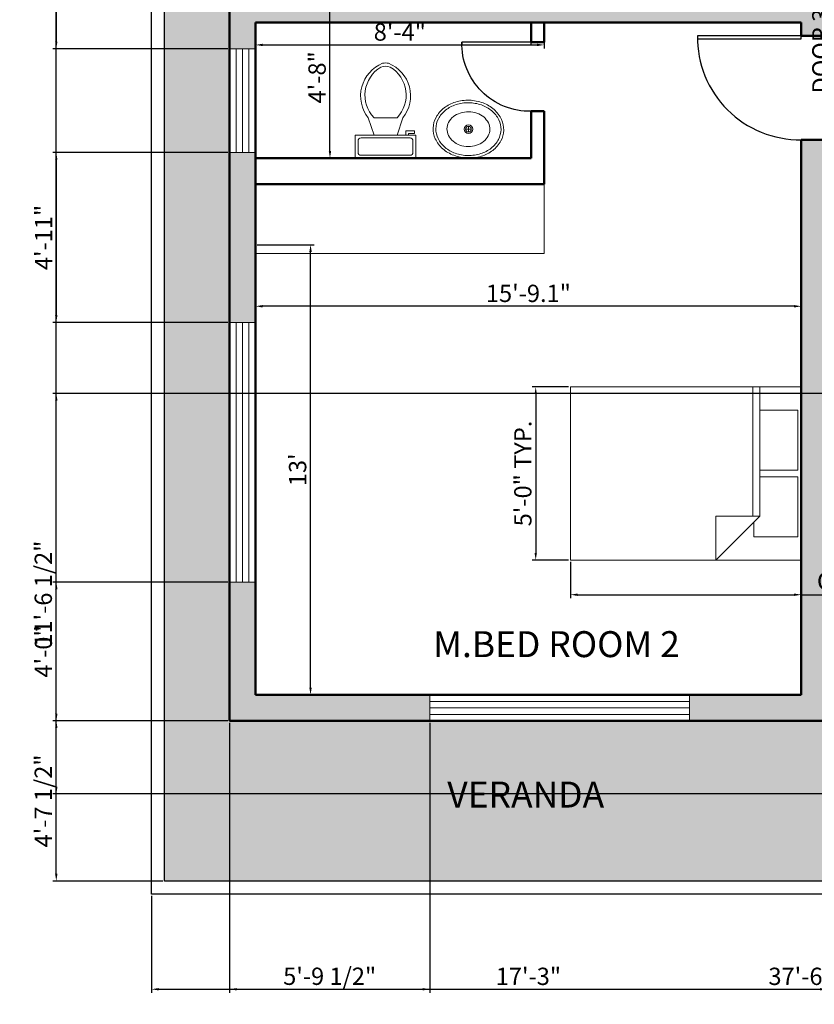
# Model space of a CAD drawing. Units: inches. Extents: x 2623 to 3157, y 1514 to 2273.
# Tile 1 of 6: x 2623 to 2898, y 1514 to 1856. Entities that reach past the tile are written whole.
import ezdxf

# ---------------------------------------------------------------- set-up
doc = ezdxf.new("R2010")
doc.units = ezdxf.units.IN
for name, color, linetype, lineweight in [('A-ANNO-DIMS', 2, 'Continuous', 18), ('A-AREA-IDEN', 7, 'Continuous', 25), ('A-DOOR', 4, 'Continuous', 25), ('A-FLOR-CASE', 8, 'Continuous', 20), ('A-FLOR-FIXT', 9, 'Continuous', 18), ('A-FURN', 8, 'Continuous', 18), ('A-GLAZ', 4, 'Continuous', 20), ('A-WALL', 7, 'Continuous', 50), ('A-WALL-PATT', 252, 'Continuous', 13), ('C-PROP', 7, 'Continuous', 25), ('L-PLNT-PATT', 9, 'Continuous', 13)]:
    doc.layers.add(name, color=color, linetype=linetype, lineweight=lineweight)
doc.styles.get("Standard").update_dxf_attribs({"font": 'arial.ttf'})
doc.dimstyles.new('ISO-25', dxfattribs={"dimtxt": 6, "dimasz": 2.5, "dimexe": 1.25, "dimexo": 0.625, "dimtad": 1, "dimdec": 1, "dimlunit": 3, "dimtxsty": 'Standard', "dimcen": 2.5, "dimadec": 0, "dimazin": 0, "dimtfac": 1, "dimtdec": 1, "dimtmove": 0, "dimatfit": 3, "dimfxl": 1, "dimarcsym": 0})

# ---------------------------------------------------------------- blocks, each defined once
blk = doc.blocks.new('Bed - Queen')
for p, q in [((0, -80.00003), (0, 0)), ((0, 0), (59.99999, 0)), ((59.99999, 0), (59.99999, -80.00003)), ((7.99999, -1.2), (28.79998, -1.2)), ((7.99999, -14.4), (7.99999, -1.2)), ((28.79998, -1.2), (28.79998, -14.4)), ((31.19999, -1.2), (51.99999, -1.2)), ((31.19999, -14.4), (31.19999, -1.2)), ((51.99999, -1.2), (51.99999, -16.4)), ((0, -14.4), (44.8, -14.4)), ((44.8, -16.8), (0, -16.8)), ((59.99999, -29.6), (44.8, -14.4)), ((44.8, -14.4), (44.8, -29.6)), ((51.99999, -16.4), (46.79936, -16.4)), ((44.8, -29.6), (59.99999, -29.6)), ((59.99999, -80.00003), (0, -80.00003))]:
    blk.add_line(p, q)
blk = doc.blocks.new('Toilet - top')
for p, q in [((9.5, -6), (9.5, -2)), ((-10, -8.5), (-8, -8.5)), ((-10, -9.5), (-10, -8.5)), ((-7, -9.5), (-10, -9.5)), ((-8, -8.5), (-8, -8)), ((-7, -8), (-7, -9.5)), ((-4, -8), (-6, -14)), ((4, -8), (6, -14)), ((4, -14), (-4, -14))]:
    blk.add_line(p, q)
blk.add_lwpolyline([(10.5, -8), (10.5, 0), (-10.5, 0), (-10.5, -8)], close=True)
for points in [[(-9.5, -2), (-9.5, -6)], [(8.5, -1), (-8.5, -1)], [(-8.5, -7), (8.5, -7)]]:
    blk.add_lwpolyline(points)
for centre, radius, start, end in [((-8.62, -1.88), 0.884, 81.8699, 188.1301), ((8.62, -1.88), 0.884, 351.8699, 98.1301), ((-8.62, -6.12), 0.884, 171.8699, 278.1301), ((8.62, -6.12), 0.884, 261.8699, 8.1301), ((3.52, -21.58), 12.17, 141.4691, 247.9714), ((4.2, -21.82), 11.33, 136.3677, 238.9468), ((-3.52, -21.58), 12.17, 292.0284, 38.5307), ((-4.2, -21.82), 11.33, 301.053, 43.6321), ((0, -27.88), 4, 245.7318, 294.2682), ((0, -29), 4, 254.8605, 285.1395)]:
    blk.add_arc(centre, radius, start, end)
blk = doc.blocks.new('Sink - Oval top')
for p, q in [((-1, 0), (1, 0)), ((0, 1), (0, -1))]:
    blk.add_line(p, q)
for points in [[(-12.23, 0.39, 0.117634), (-11.46, -3.36, 0.104469), (-8.88, -6.8, 0.090016), (-5.08, -9.07, 0.08192), (-0.32, -10.02, 0.08192), (4.49, -9.38, 0.090016), (8.42, -7.36, 0.104469), (11.22, -4.09, 0.117634), (12.23, -0.39, 0.117634), (11.46, 3.36, 0.104469), (8.88, 6.8, 0.090016), (5.08, 9.07, 0.08192), (0.32, 10.02, 0.08192), (-4.49, 9.38, 0.090016), (-8.42, 7.36, 0.104469), (-11.22, 4.09, 0.117634)], [(-11.29, 0.16, 0.118622), (-10.52, -3.25, 0.104678), (-8.07, -6.36, 0.089562), (-4.54, -8.37, 0.081185), (-0.13, -9.15, 0.081185), (4.3, -8.49, 0.089562), (7.89, -6.58, 0.104678), (10.42, -3.55, 0.118622), (11.29, -0.16, 0.118622), (10.52, 3.25, 0.104678), (8.07, 6.36, 0.089562), (4.54, 8.37, 0.081185), (0.13, 9.15, 0.081185), (-4.3, 8.49, 0.089562), (-7.89, 6.58, 0.104678), (-10.42, 3.55, 0.118622)], [(-7.42, 0.08, 0.118283), (-6.91, -2.17, 0.104607), (-5.29, -4.21, 0.089718), (-2.97, -5.53, 0.081436), (-0.07, -6.04, 0.081436), (2.84, -5.59, 0.089718), (5.2, -4.33, 0.104607), (6.86, -2.32, 0.118283), (7.42, -0.08, 0.118283), (6.91, 2.17, 0.104607), (5.29, 4.21, 0.089718), (2.97, 5.53, 0.081436), (0.07, 6.04, 0.081436), (-2.84, 5.59, 0.089718), (-5.2, 4.33, 0.104607), (-6.86, 2.32, 0.118283)]]:
    blk.add_lwpolyline(points, format="xyb", close=True)
for radius in [1.5, 1]:
    blk.add_circle((0, 0), radius)
blk = doc.blocks.new('Window - Wood Frame 36 in. Wide plan')
for p, q in [((0, 6), (0, 0)), ((36, 6), (36, 0)), ((0, 4.5), (36, 4.5)), ((0, 3), (36, 3)), ((0, 1.5), (36, 1.5))]:
    blk.add_line(p, q)
blk = doc.blocks.new('*D24')
at = {"layer": 'A-ANNO-DIMS', "color": 0, "lineweight": -2, "transparency": 16777216}
for p, q in [((2704.92, 1777.65), (2724.62, 1777.65)), ((2723.37, 1624.15), (2723.37, 1775.15)), ((2704.92, 1621.65), (2724.62, 1621.65))]:
    blk.add_line(p, q, dxfattribs=at)
at = {"layer": 'A-ANNO-DIMS', "color": 0, "transparency": 16777216}
for points in [[(2722.95, 1775.15), (2723.79, 1775.15), (2723.37, 1777.65)], [(2722.95, 1624.15), (2723.79, 1624.15), (2723.37, 1621.65)]]:
    blk.add_solid(points, dxfattribs=at)
at = {"layer": 'Defpoints', "color": 0, "transparency": 16777216}
for p in [(2704.3, 1777.65), (2723.37, 1777.65), (2704.3, 1621.65)]:
    blk.add_point(p, dxfattribs=at)
at = {"layer": 'A-ANNO-DIMS', "color": 0, "transparency": 16777216, "insert": (2719.68, 1699.65), "char_height": 6, "attachment_point": 5, "rotation": 90}
blk.add_mtext("13'", dxfattribs=at)
blk = doc.blocks.new('*D25')
at = {"layer": 'A-ANNO-DIMS', "color": 0, "lineweight": -2, "transparency": 16777216}
for p, q in [((2704.3, 1622.27), (2704.3, 1757.57)), ((2893.38, 1622.27), (2893.38, 1757.57)), ((2890.88, 1756.32), (2706.8, 1756.32))]:
    blk.add_line(p, q, dxfattribs=at)
at = {"layer": 'A-ANNO-DIMS', "color": 0, "transparency": 16777216}
for points in [[(2706.8, 1756.74), (2706.8, 1755.9), (2704.3, 1756.32)], [(2890.88, 1756.74), (2890.88, 1755.9), (2893.38, 1756.32)]]:
    blk.add_solid(points, dxfattribs=at)
at = {"layer": 'Defpoints', "color": 0, "transparency": 16777216}
for p in [(2704.3, 1756.32), (2704.3, 1621.65), (2893.38, 1621.65)]:
    blk.add_point(p, dxfattribs=at)
at = {"layer": 'A-ANNO-DIMS', "color": 0, "transparency": 16777216, "insert": (2798.84, 1760.01), "char_height": 6, "attachment_point": 5}
blk.add_mtext('15\'-9.1"', dxfattribs=at)
blk = doc.blocks.new('*D26')
at = {"layer": 'A-ANNO-DIMS', "color": 0, "lineweight": -2, "transparency": 16777216}
for p, q in [((2704.3, 1854.02), (2704.3, 1845.64)), ((2804.3, 1854.02), (2804.3, 1845.64)), ((2706.8, 1846.89), (2801.8, 1846.89))]:
    blk.add_line(p, q, dxfattribs=at)
at = {"layer": 'A-ANNO-DIMS', "color": 0, "transparency": 16777216}
for points in [[(2706.8, 1847.31), (2706.8, 1846.48), (2704.3, 1846.89)], [(2801.8, 1847.31), (2801.8, 1846.48), (2804.3, 1846.89)]]:
    blk.add_solid(points, dxfattribs=at)
at = {"layer": 'Defpoints', "color": 0, "transparency": 16777216}
for p in [(2704.3, 1854.65), (2804.3, 1854.65), (2804.3, 1846.89)]:
    blk.add_point(p, dxfattribs=at)
at = {"layer": 'A-ANNO-DIMS', "color": 0, "transparency": 16777216, "insert": (2754.3, 1850.58), "char_height": 6, "attachment_point": 5}
blk.add_mtext('8\'-4"', dxfattribs=at)
blk = doc.blocks.new('*D27')
at = {"layer": 'A-ANNO-DIMS', "color": 0, "lineweight": -2, "transparency": 16777216}
for p, q in [((2704.92, 1863.65), (2731.35, 1863.65)), ((2730.1, 1810.15), (2730.1, 1861.15)), ((2704.92, 1807.65), (2731.35, 1807.65))]:
    blk.add_line(p, q, dxfattribs=at)
at = {"layer": 'A-ANNO-DIMS', "color": 0, "transparency": 16777216}
for points in [[(2729.68, 1861.15), (2730.51, 1861.15), (2730.1, 1863.65)], [(2729.68, 1810.15), (2730.51, 1810.15), (2730.1, 1807.65)]]:
    blk.add_solid(points, dxfattribs=at)
at = {"layer": 'Defpoints', "color": 0, "transparency": 16777216}
for p in [(2704.3, 1863.65), (2730.1, 1863.65), (2704.3, 1807.65)]:
    blk.add_point(p, dxfattribs=at)
at = {"layer": 'A-ANNO-DIMS', "color": 0, "transparency": 16777216, "insert": (2726.41, 1835.65), "char_height": 6, "attachment_point": 5, "rotation": 90}
blk.add_mtext('4\'-8"', dxfattribs=at)
blk = doc.blocks.new('DOOR-SWING-24IN')
for p, q in [((0, 0), (0, 1)), ((0, 1), (24, 1)), ((24, 0), (0, 0)), ((24, 1), (24, 0))]:
    blk.add_line(p, q)
blk.add_arc((23.5, 0.5), 23.51, 88.7811, 181.2189)
blk = doc.blocks.new('DOOR-SWING-36IN')
for p, q in [((36, 1), (0, 1)), ((0, 1), (0, 0)), ((36, 0), (36, 1)), ((0, 0), (36, 0))]:
    blk.add_line(p, q)
blk.add_arc((0.5, 0.5), 35.5, 359.1931, 90.8069)
blk = doc.blocks.new('*D39')
at = {"layer": 'A-ANNO-DIMS', "color": 0, "lineweight": -2, "transparency": 16777216}
for p, q in [((2904.66, 1825.78), (2904.66, 1893.28)), ((2909.45, 1825.78), (2903.41, 1825.78)), ((2904.66, 1792.15), (2904.66, 1823.28)), ((2909.45, 1789.65), (2903.41, 1789.65))]:
    blk.add_line(p, q, dxfattribs=at)
at = {"layer": 'A-ANNO-DIMS', "color": 0, "transparency": 16777216}
for points in [[(2904.24, 1823.28), (2905.08, 1823.28), (2904.66, 1825.78)], [(2904.24, 1792.15), (2905.08, 1792.15), (2904.66, 1789.65)]]:
    blk.add_solid(points, dxfattribs=at)
at = {"layer": 'Defpoints', "color": 0, "transparency": 16777216}
for p in [(2904.66, 1825.78), (2910.08, 1825.78), (2910.08, 1789.65)]:
    blk.add_point(p, dxfattribs=at)
at = {"layer": 'A-ANNO-DIMS', "color": 0, "transparency": 16777216, "insert": (2900.93, 1860.78), "char_height": 6, "attachment_point": 5, "rotation": 90}
blk.add_mtext('DOOR 3\'-0" TYP.', dxfattribs=at)
blk = doc.blocks.new('*D41')
at = {"layer": 'A-ANNO-DIMS', "color": 0, "lineweight": -2, "transparency": 16777216}
for p, q in [((2813.38, 1667.74), (2813.38, 1655.12)), ((2893.38, 1667.74), (2893.38, 1655.12)), ((2815.88, 1656.37), (2890.88, 1656.37)), ((2893.38, 1656.37), (2985.39, 1656.37))]:
    blk.add_line(p, q, dxfattribs=at)
at = {"layer": 'A-ANNO-DIMS', "color": 0, "transparency": 16777216}
for points in [[(2815.88, 1656.78), (2815.88, 1655.95), (2813.38, 1656.37)], [(2890.88, 1656.78), (2890.88, 1655.95), (2893.38, 1656.37)]]:
    blk.add_solid(points, dxfattribs=at)
at = {"layer": 'Defpoints', "color": 0, "transparency": 16777216}
for p in [(2813.38, 1668.37), (2893.38, 1668.37), (2893.38, 1656.37)]:
    blk.add_point(p, dxfattribs=at)
at = {"layer": 'A-ANNO-DIMS', "color": 0, "transparency": 16777216, "insert": (2940.63, 1660.28), "char_height": 6, "attachment_point": 5}
blk.add_mtext('QUEEN BED 6\'-8" TYP.', dxfattribs=at)
blk = doc.blocks.new('*D42')
at = {"layer": 'A-ANNO-DIMS', "color": 0, "lineweight": -2, "transparency": 16777216}
for p, q in [((2812.75, 1728.37), (2800.13, 1728.37)), ((2801.38, 1725.87), (2801.38, 1670.87)), ((2812.75, 1668.37), (2800.13, 1668.37))]:
    blk.add_line(p, q, dxfattribs=at)
at = {"layer": 'A-ANNO-DIMS', "color": 0, "transparency": 16777216}
for points in [[(2800.96, 1725.87), (2801.79, 1725.87), (2801.38, 1728.37)], [(2800.96, 1670.87), (2801.79, 1670.87), (2801.38, 1668.37)]]:
    blk.add_solid(points, dxfattribs=at)
at = {"layer": 'Defpoints', "color": 0, "transparency": 16777216}
for p in [(2813.38, 1728.37), (2801.38, 1668.37), (2813.38, 1668.37)]:
    blk.add_point(p, dxfattribs=at)
at = {"layer": 'A-ANNO-DIMS', "color": 0, "transparency": 16777216, "insert": (2797.69, 1698.37), "char_height": 6, "attachment_point": 5, "rotation": 90}
blk.add_mtext('5\'-0" TYP.', dxfattribs=at)
blk = doc.blocks.new('*D59')
at = {"layer": 'A-ANNO-DIMS', "color": 0, "lineweight": -2, "transparency": 16777216}
for p, q in [((2668.3, 1552.02), (2668.3, 1518.4)), ((3118.3, 1552.02), (3118.3, 1518.4)), ((2670.8, 1519.65), (3115.8, 1519.65))]:
    blk.add_line(p, q, dxfattribs=at)
at = {"layer": 'A-ANNO-DIMS', "color": 0, "transparency": 16777216}
for points in [[(2670.8, 1520.06), (2670.8, 1519.23), (2668.3, 1519.65)], [(3115.8, 1520.06), (3115.8, 1519.23), (3118.3, 1519.65)]]:
    blk.add_solid(points, dxfattribs=at)
at = {"layer": 'Defpoints', "color": 0, "transparency": 16777216}
for p in [(2668.3, 1552.65), (3118.3, 1552.65), (3118.3, 1519.65)]:
    blk.add_point(p, dxfattribs=at)
at = {"layer": 'A-ANNO-DIMS', "color": 0, "transparency": 16777216, "insert": (2893.3, 1523.34), "char_height": 6, "attachment_point": 5}
blk.add_mtext('37\'-6"', dxfattribs=at)
blk = doc.blocks.new('*D62')
at = {"layer": 'A-ANNO-DIMS', "color": 0, "lineweight": -2, "transparency": 16777216}
for p, q in [((2694.67, 2185.65), (2634.05, 2185.65)), ((2635.3, 1615.15), (2635.3, 2183.15)), ((2694.67, 1612.65), (2634.05, 1612.65))]:
    blk.add_line(p, q, dxfattribs=at)
at = {"layer": 'A-ANNO-DIMS', "color": 0, "transparency": 16777216}
for points in [[(2634.88, 2183.15), (2635.71, 2183.15), (2635.3, 2185.65)], [(2634.88, 1615.15), (2635.71, 1615.15), (2635.3, 1612.65)]]:
    blk.add_solid(points, dxfattribs=at)
at = {"layer": 'Defpoints', "color": 0, "transparency": 16777216}
for p in [(2635.3, 2185.65), (2695.3, 2185.65), (2695.3, 1612.65)]:
    blk.add_point(p, dxfattribs=at)
at = {"layer": 'A-ANNO-DIMS', "color": 0, "transparency": 16777216, "insert": (2631.61, 1899.15), "char_height": 6, "attachment_point": 5, "rotation": 90}
blk.add_mtext('47\'-9"', dxfattribs=at)
blk = doc.blocks.new('*D65')
at = {"layer": 'A-ANNO-DIMS', "color": 0, "lineweight": -2, "transparency": 16777216}
for p, q in [((2695.3, 1612.02), (2695.3, 1518.4)), ((2902.38, 1612.02), (2902.38, 1518.4)), ((2697.8, 1519.65), (2899.88, 1519.65))]:
    blk.add_line(p, q, dxfattribs=at)
at = {"layer": 'A-ANNO-DIMS', "color": 0, "transparency": 16777216}
for points in [[(2697.8, 1520.06), (2697.8, 1519.23), (2695.3, 1519.65)], [(2899.88, 1520.06), (2899.88, 1519.23), (2902.38, 1519.65)]]:
    blk.add_solid(points, dxfattribs=at)
at = {"layer": 'Defpoints', "color": 0, "transparency": 16777216}
for p in [(2695.3, 1612.65), (2902.38, 1612.65), (2902.38, 1519.65)]:
    blk.add_point(p, dxfattribs=at)
at = {"layer": 'A-ANNO-DIMS', "color": 0, "transparency": 16777216, "insert": (2798.84, 1523.34), "char_height": 6, "attachment_point": 5}
blk.add_mtext('17\'-3"', dxfattribs=at)
blk = doc.blocks.new('*D68')
at = {"layer": 'A-ANNO-DIMS', "color": 0, "lineweight": -2, "transparency": 16777216}
for p, q in [((2994.24, 1726.09), (2634.05, 1726.09)), ((2635.3, 1589.88), (2635.3, 1723.59)), ((2994.24, 1587.38), (2634.05, 1587.38))]:
    blk.add_line(p, q, dxfattribs=at)
at = {"layer": 'A-ANNO-DIMS', "color": 0, "transparency": 16777216}
for points in [[(2634.88, 1723.59), (2635.71, 1723.59), (2635.3, 1726.09)], [(2634.88, 1589.88), (2635.71, 1589.88), (2635.3, 1587.38)]]:
    blk.add_solid(points, dxfattribs=at)
at = {"layer": 'Defpoints', "color": 0, "transparency": 16777216}
for p in [(2635.3, 1726.09), (2994.86, 1726.09), (2994.86, 1587.38)]:
    blk.add_point(p, dxfattribs=at)
at = {"layer": 'A-ANNO-DIMS', "color": 0, "transparency": 16777216, "insert": (2631.57, 1656.73), "char_height": 6, "attachment_point": 5, "rotation": 90}
blk.add_mtext('11\'-6 1/2"', dxfattribs=at)
blk = doc.blocks.new('*D79')
at = {"layer": 'A-ANNO-DIMS', "color": 0, "lineweight": -2, "transparency": 16777216}
for p, q in [((2695.3, 1612.02), (2695.3, 1518.4)), ((2764.7, 1612.02), (2764.7, 1518.4)), ((2697.8, 1519.65), (2762.2, 1519.65))]:
    blk.add_line(p, q, dxfattribs=at)
at = {"layer": 'A-ANNO-DIMS', "color": 0, "transparency": 16777216}
for points in [[(2697.8, 1520.06), (2697.8, 1519.23), (2695.3, 1519.65)], [(2762.2, 1520.06), (2762.2, 1519.23), (2764.7, 1519.65)]]:
    blk.add_solid(points, dxfattribs=at)
at = {"layer": 'Defpoints', "color": 0, "transparency": 16777216}
for p in [(2695.3, 1612.65), (2764.7, 1612.65), (2764.7, 1519.65)]:
    blk.add_point(p, dxfattribs=at)
at = {"layer": 'A-ANNO-DIMS', "color": 0, "transparency": 16777216, "insert": (2730, 1523.37), "char_height": 6, "attachment_point": 5}
blk.add_mtext('5\'-9 1/2"', dxfattribs=at)
blk = doc.blocks.new('*D80')
at = {"layer": 'A-ANNO-DIMS', "color": 0, "lineweight": -2, "transparency": 16777216}
for p, q in [((2694.67, 1660.74), (2634.05, 1660.74)), ((2635.3, 1615.15), (2635.3, 1658.24)), ((2694.67, 1612.65), (2634.05, 1612.65))]:
    blk.add_line(p, q, dxfattribs=at)
at = {"layer": 'A-ANNO-DIMS', "color": 0, "transparency": 16777216}
for points in [[(2634.88, 1658.24), (2635.71, 1658.24), (2635.3, 1660.74)], [(2634.88, 1615.15), (2635.71, 1615.15), (2635.3, 1612.65)]]:
    blk.add_solid(points, dxfattribs=at)
at = {"layer": 'Defpoints', "color": 0, "transparency": 16777216}
for p in [(2635.3, 1660.74), (2695.3, 1660.74), (2695.3, 1612.65)]:
    blk.add_point(p, dxfattribs=at)
at = {"layer": 'A-ANNO-DIMS', "color": 0, "transparency": 16777216, "insert": (2631.61, 1636.69), "char_height": 6, "attachment_point": 5, "rotation": 90}
blk.add_mtext('4\'-0"', dxfattribs=at)
blk = doc.blocks.new('*D88')
at = {"layer": 'A-ANNO-DIMS', "color": 0, "lineweight": -2, "transparency": 16777216}
for p, q in [((2694.67, 1612.65), (2634.05, 1612.65)), ((2635.3, 1559.65), (2635.3, 1610.15)), ((2672.17, 1557.15), (2634.05, 1557.15))]:
    blk.add_line(p, q, dxfattribs=at)
at = {"layer": 'A-ANNO-DIMS', "color": 0, "transparency": 16777216}
for points in [[(2634.88, 1610.15), (2635.71, 1610.15), (2635.3, 1612.65)], [(2634.88, 1559.65), (2635.71, 1559.65), (2635.3, 1557.15)]]:
    blk.add_solid(points, dxfattribs=at)
at = {"layer": 'Defpoints', "color": 0, "transparency": 16777216}
for p in [(2635.3, 1612.65), (2695.3, 1612.65), (2672.8, 1557.15)]:
    blk.add_point(p, dxfattribs=at)
at = {"layer": 'A-ANNO-DIMS', "color": 0, "transparency": 16777216, "insert": (2631.57, 1584.9), "char_height": 6, "attachment_point": 5, "rotation": 90}
blk.add_mtext('4\'-7 1/2"', dxfattribs=at)
blk = doc.blocks.new('*D90')
at = {"layer": 'A-ANNO-DIMS', "color": 0, "lineweight": -2, "transparency": 16777216}
for p, q in [((2694.67, 1949.25), (2634.05, 1949.25)), ((2635.3, 1946.75), (2635.3, 1848.07)), ((2694.67, 1845.57), (2634.05, 1845.57))]:
    blk.add_line(p, q, dxfattribs=at)
at = {"layer": 'A-ANNO-DIMS', "color": 0, "transparency": 16777216}
for points in [[(2634.88, 1946.75), (2635.71, 1946.75), (2635.3, 1949.25)], [(2634.88, 1848.07), (2635.71, 1848.07), (2635.3, 1845.57)]]:
    blk.add_solid(points, dxfattribs=at)
at = {"layer": 'Defpoints', "color": 0, "transparency": 16777216}
for p in [(2695.3, 1949.25), (2635.3, 1845.57), (2695.3, 1845.57)]:
    blk.add_point(p, dxfattribs=at)
at = {"layer": 'A-ANNO-DIMS', "color": 0, "transparency": 16777216, "insert": (2631.57, 1897.41), "char_height": 6, "attachment_point": 5, "rotation": 90}
blk.add_mtext('8\'-7 1/2"', dxfattribs=at)
blk = doc.blocks.new('*D91')
at = {"layer": 'A-ANNO-DIMS', "color": 0, "lineweight": -2, "transparency": 16777216}
for p, q in [((2694.67, 1809.57), (2634.05, 1809.57)), ((2635.3, 1807.07), (2635.3, 1753.24)), ((2694.67, 1750.74), (2634.05, 1750.74))]:
    blk.add_line(p, q, dxfattribs=at)
at = {"layer": 'A-ANNO-DIMS', "color": 0, "transparency": 16777216}
for points in [[(2634.88, 1807.07), (2635.71, 1807.07), (2635.3, 1809.57)], [(2634.88, 1753.24), (2635.71, 1753.24), (2635.3, 1750.74)]]:
    blk.add_solid(points, dxfattribs=at)
at = {"layer": 'Defpoints', "color": 0, "transparency": 16777216}
for p in [(2695.3, 1809.57), (2635.3, 1750.74), (2695.3, 1750.74)]:
    blk.add_point(p, dxfattribs=at)
at = {"layer": 'A-ANNO-DIMS', "color": 0, "transparency": 16777216, "insert": (2631.66, 1780.16), "char_height": 6, "attachment_point": 5, "rotation": 90}
blk.add_mtext('4\'-11"', dxfattribs=at)

msp = doc.modelspace()

# ---------------------------------------------------------------- hatches: boundary and pattern name
at = {"layer": 'A-WALL-PATT'}
h = msp.add_hatch(color=256, dxfattribs=at)
h.dxf.hatch_style = 1
h.paths.add_polyline_path([(2704.3, 1854.65), (2893.38, 1854.65), (2893.38, 1850.02), (2902.38, 1850.02), (2902.38, 1863.65), (2704.3, 1863.65), (2704.3, 1949.25), (2695.3, 1949.25), (2695.3, 1845.57), (2704.3, 1845.57)])
h.paths.add_polyline_path([(2704.3, 1809.57), (2695.3, 1809.57), (2695.3, 1750.74), (2704.3, 1750.74)])
h.paths.add_polyline_path([(2764.7, 1621.65), (2704.3, 1621.65), (2704.3, 1660.74), (2695.3, 1660.74), (2695.3, 1612.65), (2764.7, 1612.65)])
h.paths.add_polyline_path([(2704.3, 2128.1), (2695.3, 2128.1), (2695.3, 2039.25), (2704.3, 2039.25)])
h.paths.add_polyline_path([(2714, 2185.65), (2695.3, 2185.65), (2695.3, 2164.1), (2704.3, 2164.1), (2704.3, 2176.65), (2714, 2176.65)])
h.paths.add_polyline_path([(2797.66, 2185.65), (2768, 2185.65), (2768, 2176.65), (2797.66, 2176.65)])
h.paths.add_polyline_path([(2777.8, 2176.65), (2773.3, 2176.65), (2773.3, 2142.65), (2777.8, 2142.65)])
h.paths.add_polyline_path([(2963.13, 2185.65), (2887.66, 2185.65), (2887.66, 2176.65), (2963.13, 2176.65)])
h.paths.add_polyline_path([(2928.3, 2176.65), (2919.3, 2176.65), (2919.3, 2047.65), (2850.8, 2047.65), (2850.8, 2038.65), (2919.3, 2038.65), (2919.3, 2031.57), (2928.3, 2031.57), (2928.3, 2038.65)])
h.paths.add_polyline_path([(3082.3, 2185.65), (3053.13, 2185.65), (3053.13, 2176.65), (3073.3, 2176.65), (3073.3, 2169.26), (3082.3, 2169.26)])
h.paths.add_polyline_path([(3082.3, 2133.26), (3073.3, 2133.26), (3073.3, 2047.65), (2977.8, 2047.65), (2977.8, 2074.51), (2973.3, 2074.51), (2973.3, 2047.65), (2973.3, 2038.65), (2973.3, 2021.33), (2977.8, 2021.33), (2977.8, 2038.65), (3005.74, 2038.65, -0.027912), (3007.41, 2038.69, -0.0118), (3008.11, 2038.65), (3073.3, 2038.65), (3073.3, 2034.16), (3082.3, 2034.16)])
h.paths.add_polyline_path([(3082.3, 1998.16), (3073.3, 1998.16), (3073.3, 1991.65), (2977.8, 1991.65), (2977.8, 1997.33), (2973.3, 1997.33), (2973.3, 1991.65), (2928.3, 1991.65), (2928.3, 1995.57), (2919.3, 1995.57), (2919.3, 1982.65), (3073.3, 1982.65), (3073.3, 1974.57), (3082.3, 1974.57)])
h = msp.add_hatch(color=256, dxfattribs=at)
h.dxf.hatch_style = 1
h.paths.add_polyline_path([(3082.3, 1813.09), (3073.3, 1813.09), (3073.3, 1789.65), (3059.78, 1789.65), (3059.78, 1780.65), (3082.3, 1780.65)])
h.paths.add_polyline_path([(2969.78, 1789.65), (2946.08, 1789.65), (2946.08, 1780.65), (2969.78, 1780.65)])
h.paths.add_polyline_path([(2910.08, 1789.65), (2902.38, 1789.65), (2902.38, 1814.02), (2893.38, 1814.02), (2893.38, 1621.65), (2854.7, 1621.65), (2854.7, 1612.65), (2902.38, 1612.65), (2902.38, 1780.65), (2910.08, 1780.65)])
at = {"layer": 'L-PLNT-PATT'}
h = msp.add_hatch(color=256, dxfattribs=at)
h.dxf.hatch_style = 1
h.set_gradient(color1=(19, 155, 72), color2=(63, 255, 0), name='CURVED')
h.paths.add_polyline_path([(2902.38, 1612.65), (2695.3, 1612.65), (2695.3, 2185.65), (3082.3, 2185.65), (3082.3, 1780.65), (3113.8, 1780.65), (3113.8, 2208.15), (2672.8, 2208.15), (2672.8, 1557.15), (2902.38, 1557.15)])
h = msp.add_hatch(color=256, dxfattribs=at)
h.dxf.hatch_style = 1
h.set_gradient(color1=(19, 155, 72), color2=(63, 255, 0), name='CYLINDER')
h.paths.add_polyline_path([(3024.32, 1726.09), (2994.86, 1726.09), (2994.86, 1587.38), (3024.32, 1587.38)], flags=17)
h.paths.add_polyline_path([(2902.38, 1612.65), (2695.3, 1612.65), (2695.3, 2185.65), (3082.3, 2185.65), (3082.3, 1780.65), (3113.8, 1780.65), (3113.8, 2208.15), (2672.8, 2208.15), (2672.8, 1557.15), (2902.38, 1557.15)])

# ---------------------------------------------------------------- linework, layer by layer
at = {"layer": 'A-FLOR-CASE'}
for p, q in [((2804.3, 1798.65), (2804.3, 1774.65)), ((2804.3, 1774.65), (2704.3, 1774.65))]:
    msp.add_line(p, q, dxfattribs=at)
at = {"layer": 'A-GLAZ'}
for p, q in [((2704.3, 1845.57), (2695.3, 1845.57)), ((2695.3, 1809.57), (2704.3, 1809.57)), ((2695.3, 1750.74), (2704.3, 1750.74)), ((2704.3, 1660.74), (2695.3, 1660.74)), ((2764.7, 1621.65), (2764.7, 1612.65)), ((2854.7, 1621.65), (2854.7, 1612.65))]:
    msp.add_line(p, q, dxfattribs=at)
at = {"layer": 'A-WALL'}
for p, q in [((2695.3, 1612.65), (2695.3, 2185.65)), ((2704.3, 1621.65), (2704.3, 1854.65)), ((2704.3, 1854.65), (2893.38, 1854.65)), ((2799.8, 1847.89), (2799.8, 1854.65)), ((2804.3, 1847.89), (2804.3, 1854.65)), ((2893.38, 1850.02), (2893.38, 1854.65)), ((2893.38, 1850.02), (2902.38, 1850.02)), ((2799.8, 1847.89), (2804.3, 1847.89)), ((2799.8, 1807.65), (2799.8, 1823.89)), ((2804.3, 1823.89), (2799.8, 1823.89)), ((2804.3, 1798.65), (2804.3, 1823.89)), ((2893.38, 1621.65), (2893.38, 1814.02)), ((2902.38, 1814.02), (2893.38, 1814.02)), ((2704.3, 1807.65), (2799.8, 1807.65)), ((2704.3, 1798.65), (2804.3, 1798.65)), ((2893.38, 1621.65), (2704.3, 1621.65)), ((2902.38, 1612.65), (2695.3, 1612.65))]:
    msp.add_line(p, q, dxfattribs=at)
at = {"layer": 'C-PROP'}
for p, q in [((2668.3, 1552.65), (2668.3, 2212.65)), ((2672.8, 1557.15), (2672.8, 2208.15)), ((2935.08, 1557.15), (2672.8, 1557.15)), ((2935.08, 1552.65), (2668.3, 1552.65))]:
    msp.add_line(p, q, dxfattribs=at)

# ---------------------------------------------------------------- block references
at = {"layer": 'A-DOOR', "rotation": 180}
msp.add_blockref('DOOR-SWING-36IN', (2893.38, 1850.02), dxfattribs=at)
at = {"layer": 'A-DOOR', "extrusion": (0, 0, -1), "zscale": -1, "rotation": 180}
msp.add_blockref('DOOR-SWING-24IN', (-2775.79, 1847.89), dxfattribs=at)
at = {"layer": 'A-FLOR-FIXT', "rotation": 180}
msp.add_blockref('Toilet - top', (2749.36, 1807.65), dxfattribs=at)
at = {"layer": 'A-FLOR-FIXT'}
msp.add_blockref('Sink - Oval top', (2778.06, 1817.7), dxfattribs=at)
at = {"layer": 'A-FURN', "rotation": 270}
msp.add_blockref('Bed - Queen', (2893.38, 1728.37), dxfattribs=at)
at = {"layer": 'A-GLAZ', "yscale": 1.5, "rotation": 90}
msp.add_blockref('Window - Wood Frame 36 in. Wide plan', (2704.3, 1809.57), dxfattribs=at)
at = {"layer": 'A-GLAZ', "xscale": 2.5, "yscale": 1.5, "rotation": 90}
msp.add_blockref('Window - Wood Frame 36 in. Wide plan', (2704.3, 1660.74), dxfattribs=at)
at = {"layer": 'A-GLAZ', "xscale": 2.5, "yscale": 1.5}
msp.add_blockref('Window - Wood Frame 36 in. Wide plan', (2764.7, 1612.65), dxfattribs=at)

# ---------------------------------------------------------------- texts
at = {"layer": 'A-AREA-IDEN', "insert": (2765.86, 1643.73), "char_height": 9, "attachment_point": 1}
msp.add_mtext('M.BED ROOM 2', dxfattribs=at)
at = {"layer": 'A-AREA-IDEN', "insert": (2770.74, 1591.6), "char_height": 9, "width": 91.3138, "attachment_point": 1}
msp.add_mtext('VERANDA', dxfattribs=at)

# ---------------------------------------------------------------- dimensions: what is measured, and where the dimension line sits
at = {"layer": 'A-ANNO-DIMS'}
for base, p1, p2, override, picture, middle in [((2635.3, 2185.65), (2695.3, 1612.65), (2695.3, 2185.65), {"dimdec": 1, "dimlfac": 1, "dimrnd": 0, "dimzin": 1, "dimdsep": 46, "dimlunit": 4, "dimfrac": 2}, '*D62', (2631.61, 1899.15)), ((2635.3, 1845.57), (2695.3, 1949.25), (2695.3, 1845.57), {"dimdec": 1, "dimlfac": 1, "dimrnd": 0, "dimzin": 1, "dimdsep": 46, "dimlunit": 4, "dimfrac": 2}, '*D90', (2631.57, 1897.41)), ((2730.1, 1863.65), (2704.3, 1807.65), (2704.3, 1863.65), {"dimclrd": 0, "dimclre": 0, "dimclrt": 0}, '*D27', (2726.41, 1835.65)), ((2635.3, 1750.74), (2695.3, 1809.57), (2695.3, 1750.74), {"dimdec": 1, "dimlfac": 1, "dimrnd": 0, "dimzin": 1, "dimdsep": 46, "dimlunit": 4, "dimfrac": 2}, '*D91', (2631.66, 1780.16)), ((2723.37, 1777.65), (2704.3, 1621.65), (2704.3, 1777.65), {"dimclrd": 0, "dimclre": 0, "dimclrt": 0}, '*D24', (2719.68, 1699.65)), ((2635.3, 1726.09), (2994.86, 1587.38), (2994.86, 1726.09), {"dimdec": 1, "dimlfac": 1, "dimrnd": 0, "dimzin": 1, "dimdsep": 46, "dimlunit": 4, "dimfrac": 2}, '*D68', (2631.57, 1656.73)), ((2635.3, 1660.74), (2695.3, 1612.65), (2695.3, 1660.74), {"dimdec": 1, "dimlfac": 1, "dimrnd": 0, "dimzin": 1, "dimdsep": 46, "dimlunit": 4, "dimfrac": 2}, '*D80', (2631.61, 1636.69)), ((2635.3, 1612.65), (2672.8, 1557.15), (2695.3, 1612.65), {"dimdec": 1, "dimlfac": 1, "dimrnd": 0, "dimzin": 1, "dimdsep": 46, "dimlunit": 4, "dimfrac": 2}, '*D88', (2631.57, 1584.9))]:
    dim = msp.add_linear_dim(base=base, p1=p1, p2=p2, angle=90, dimstyle='ISO-25', override=override, dxfattribs=at)
    dim.commit()
    dim.dimension.update_dxf_attribs({"geometry": picture, "text_midpoint": middle})
for base, p1, p2, angle, text, picture, middle in [((2904.66, 1825.78), (2910.08, 1789.65), (2910.08, 1825.78), 90, 'DOOR <> TYP.', '*D39', (2900.93, 1860.78)), ((2801.38, 1668.37), (2813.38, 1728.37), (2813.38, 1668.37), 270, '<> TYP.', '*D42', (2797.69, 1698.37))]:
    dim = msp.add_linear_dim(base=base, p1=p1, p2=p2, angle=angle, text=text, dimstyle='ISO-25', override={"dimdec": 1, "dimlfac": 1, "dimrnd": 0, "dimzin": 1, "dimdsep": 46, "dimlunit": 4, "dimfrac": 2}, dxfattribs=at)
    dim.commit()
    dim.dimension.update_dxf_attribs({"geometry": picture, "text_midpoint": middle})
for base, p1, p2, override, picture, middle in [((2804.3, 1846.89), (2704.3, 1854.65), (2804.3, 1854.65), {"dimclrd": 0, "dimclre": 0, "dimclrt": 0}, '*D26', (2754.3, 1850.58)), ((2704.3, 1756.32), (2893.38, 1621.65), (2704.3, 1621.65), {"dimclrd": 0, "dimclre": 0, "dimclrt": 0}, '*D25', (2798.84, 1760.01)), ((2902.38, 1519.65), (2695.3, 1612.65), (2902.38, 1612.65), {"dimdec": 1, "dimlfac": 1, "dimrnd": 0, "dimzin": 1, "dimdsep": 46, "dimlunit": 4, "dimfrac": 2}, '*D65', (2798.84, 1523.34)), ((2764.7, 1519.65), (2695.3, 1612.65), (2764.7, 1612.65), {"dimdec": 1, "dimlfac": 1, "dimrnd": 0, "dimzin": 1, "dimdsep": 46, "dimlunit": 4, "dimfrac": 2}, '*D79', (2730, 1523.37)), ((3118.3, 1519.65), (2668.3, 1552.65), (3118.3, 1552.65), {"dimdec": 1, "dimlfac": 1, "dimrnd": 0, "dimzin": 1, "dimdsep": 46, "dimlunit": 4, "dimfrac": 2}, '*D59', (2893.3, 1523.34))]:
    dim = msp.add_linear_dim(base=base, p1=p1, p2=p2, dimstyle='ISO-25', override=override, dxfattribs=at)
    dim.commit()
    dim.dimension.update_dxf_attribs({"geometry": picture, "text_midpoint": middle})
dim = msp.add_linear_dim(base=(2893.38, 1656.37), p1=(2813.38, 1668.37), p2=(2893.38, 1668.37), text='QUEEN BED <> TYP.', dimstyle='ISO-25', override={"dimdec": 1, "dimlfac": 1, "dimrnd": 0, "dimzin": 1, "dimdsep": 46, "dimlunit": 4, "dimfrac": 2}, dxfattribs=at)
dim.commit()
dim.dimension.update_dxf_attribs({"geometry": '*D41', "text_midpoint": (2940.63, 1660.28)})

doc.saveas('drawing.dxf')
